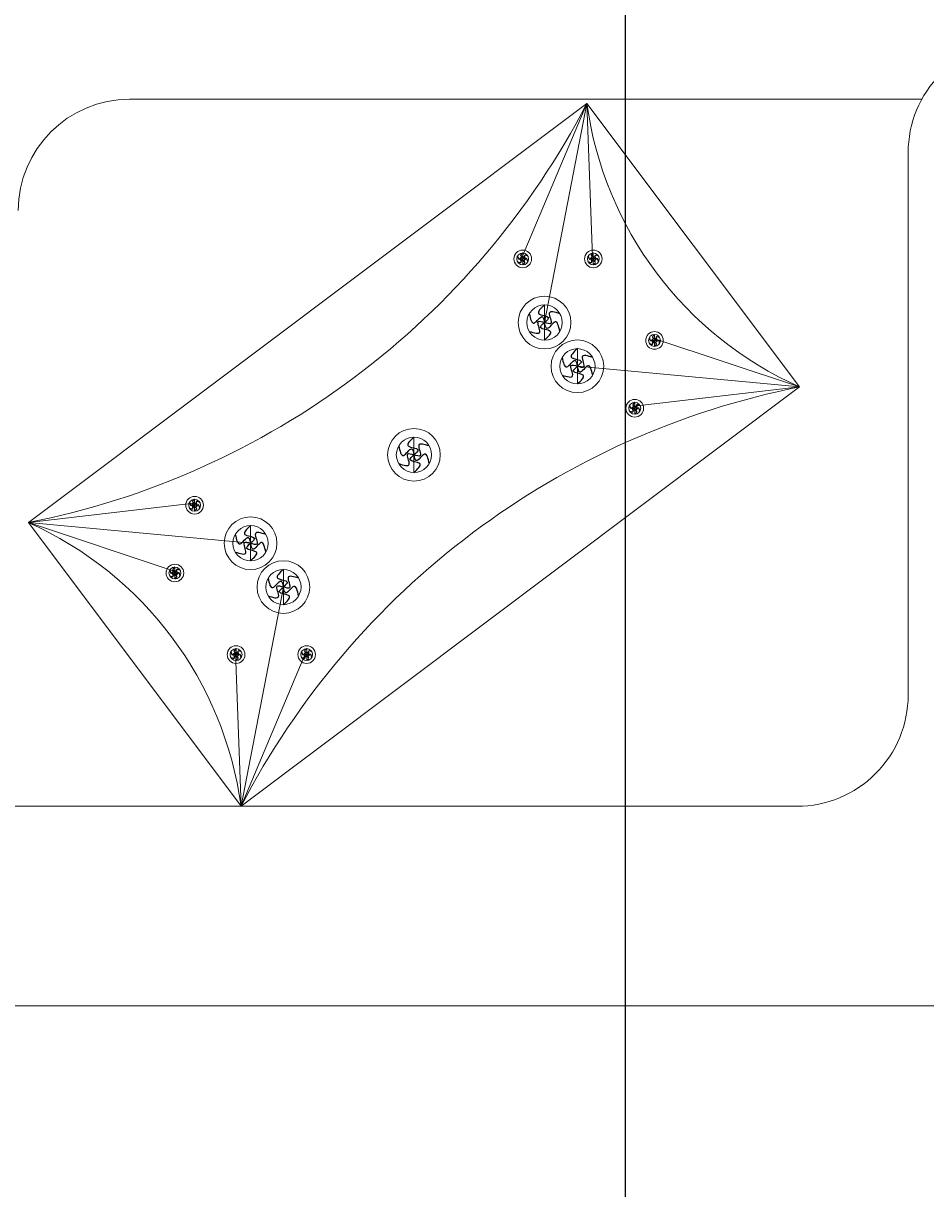
# Model space of a CAD drawing. Units: inches. Extents: x -61 to 1599, y -1316 to 257.
# Tile 107 of 204: x 200 to 224, y -166 to -135. Entities that reach past the tile are written whole.
import ezdxf

# ---------------------------------------------------------------- set-up
doc = ezdxf.new("R2010")
doc.units = ezdxf.units.IN
doc.header["$MEASUREMENT"] = 0
doc.layers.add('A-ANNO-DIMS', color=2, linetype='Continuous', lineweight=18)
doc.layers.add('FURNITURE', color=83, linetype='Continuous', lineweight=18)
doc.layers.add('FUR', color=83, linetype='Continuous')
doc.styles.get("Standard").update_dxf_attribs({"font": 'arial.ttf'})
doc.dimstyles.get("Standard").update_dxf_attribs({"dimtxt": 0.18, "dimasz": 0.18, "dimexe": 0.18, "dimexo": 0.0625, "dimgap": 0.09, "dimtad": 0, "dimtih": 1, "dimtoh": 1, "dimdec": 0, "dimzin": 0, "dimdsep": 46, "dimlunit": 3, "dimtxsty": 'Standard', "dimcen": 0.09, "dimadec": 0, "dimazin": 0, "dimtfac": 1, "dimtdec": 0, "dimtofl": 0, "dimtmove": 0, "dimatfit": 3, "dimfxl": 1, "dimtolj": 1, "dimtzin": 0, "dimarcsym": 0})

# ---------------------------------------------------------------- blocks, each defined once
blk = doc.blocks.new('*U114')
at = {"layer": 'FUR'}
blk.add_open_spline([(0.005, 0.08), (-0.03, 0.048), (-0.098, -0.015), (0.075, -0.018), (0.024, -0.063), (0.005, -0.08)], degree=3, knots=[0, 0, 0, 0, 0.0954578, 0.1898773, 0.2470677, 0.2470677, 0.2470677, 0.2470677], dxfattribs=at)
blk = doc.blocks.new('*U115')
at = {"layer": 'FUR', "transparency": 16777216}
for p, rotation in [((222.173, -79.977), 60), ((222.178, -80.056), 120), ((222.25, -80.092), 180), ((222.312, -79.968), 300), ((222.317, -80.048), 240)]:
    blk.add_blockref('*U114', p, dxfattribs=dict(at, rotation=rotation))
blk.add_blockref('*U114', (222.24, -79.932), dxfattribs=at)
blk = doc.blocks.new('*U116')
at = {"layer": 'FUR'}
blk.add_open_spline([(0.005, 0.08), (-0.03, 0.048), (-0.098, -0.015), (0.075, -0.018), (0.024, -0.063), (0.005, -0.08)], degree=3, knots=[0, 0, 0, 0, 0.0954578, 0.1898773, 0.2470677, 0.2470677, 0.2470677, 0.2470677], dxfattribs=at)
blk = doc.blocks.new('*U117')
at = {"layer": 'FUR', "transparency": 16777216}
for p, rotation in [((222.173, -79.977), 60), ((222.178, -80.056), 120), ((222.25, -80.092), 180), ((222.312, -79.968), 300), ((222.317, -80.048), 240)]:
    blk.add_blockref('*U116', p, dxfattribs=dict(at, rotation=rotation))
blk.add_blockref('*U116', (222.24, -79.932), dxfattribs=at)
blk = doc.blocks.new('*U112')
at = {"layer": 'FUR'}
blk.add_open_spline([(0.005, 0.08), (-0.03, 0.048), (-0.098, -0.015), (0.075, -0.018), (0.024, -0.063), (0.005, -0.08)], degree=3, knots=[0, 0, 0, 0, 0.0954578, 0.1898773, 0.2470677, 0.2470677, 0.2470677, 0.2470677], dxfattribs=at)
blk = doc.blocks.new('*U113')
at = {"layer": 'FUR', "transparency": 16777216}
for p, rotation in [((222.173, -79.977), 60), ((222.178, -80.056), 120), ((222.25, -80.092), 180), ((222.312, -79.968), 300), ((222.317, -80.048), 240)]:
    blk.add_blockref('*U112', p, dxfattribs=dict(at, rotation=rotation))
blk.add_blockref('*U112', (222.24, -79.932), dxfattribs=at)
blk = doc.blocks.new('*U142')
at = {"layer": 'FUR'}
blk.add_open_spline([(0.015, 0.238), (-0.088, 0.143), (-0.292, -0.045), (0.224, -0.053), (0.072, -0.187), (0.015, -0.238)], degree=3, knots=[0, 0, 0, 0, 0.2846533, 0.5662105, 0.736751, 0.736751, 0.736751, 0.736751], dxfattribs=at)
blk = doc.blocks.new('*U143')
at = {"layer": 'FUR', "transparency": 16777216}
blk.add_blockref('*U142', (662.716, -238.357), dxfattribs=at)
for p, rotation in [((662.517, -238.489), 60), ((662.929, -238.463), 300), ((662.944, -238.702), 240), ((662.531, -238.727), 120), ((662.745, -238.833), 180)]:
    blk.add_blockref('*U142', p, dxfattribs=dict(at, rotation=rotation))
blk = doc.blocks.new('*U158')
at = {"layer": 'FUR'}
blk.add_open_spline([(0.015, 0.238), (-0.088, 0.143), (-0.292, -0.045), (0.224, -0.053), (0.072, -0.187), (0.015, -0.238)], degree=3, knots=[0, 0, 0, 0, 0.2846533, 0.5662105, 0.736751, 0.736751, 0.736751, 0.736751], dxfattribs=at)
blk = doc.blocks.new('*U109')
at = {"layer": 'FUR', "transparency": 16777216}
blk.add_blockref('*U158', (662.716, -238.357), dxfattribs=at)
for p, rotation in [((662.517, -238.489), 60), ((662.929, -238.463), 300), ((662.944, -238.702), 240), ((662.531, -238.727), 120), ((662.745, -238.833), 180)]:
    blk.add_blockref('*U158', p, dxfattribs=dict(at, rotation=rotation))
blk = doc.blocks.new('*U110')
at = {"layer": 'FUR'}
blk.add_open_spline([(0.005, 0.08), (-0.03, 0.048), (-0.098, -0.015), (0.075, -0.018), (0.024, -0.063), (0.005, -0.08)], degree=3, knots=[0, 0, 0, 0, 0.0954578, 0.1898773, 0.2470677, 0.2470677, 0.2470677, 0.2470677], dxfattribs=at)
blk = doc.blocks.new('*U111')
at = {"layer": 'FUR', "transparency": 16777216}
for p, rotation in [((222.173, -79.977), 60), ((222.178, -80.056), 120), ((222.25, -80.092), 180), ((222.312, -79.968), 300), ((222.317, -80.048), 240)]:
    blk.add_blockref('*U110', p, dxfattribs=dict(at, rotation=rotation))
blk.add_blockref('*U110', (222.24, -79.932), dxfattribs=at)
blk = doc.blocks.new('*U156')
at = {"layer": 'FUR'}
blk.add_open_spline([(0.015, 0.238), (-0.088, 0.143), (-0.292, -0.045), (0.224, -0.053), (0.072, -0.187), (0.015, -0.238)], degree=3, knots=[0, 0, 0, 0, 0.2846533, 0.5662105, 0.736751, 0.736751, 0.736751, 0.736751], dxfattribs=at)
blk = doc.blocks.new('*U157')
at = {"layer": 'FUR', "transparency": 16777216}
blk.add_blockref('*U156', (662.716, -238.357), dxfattribs=at)
for p, rotation in [((662.517, -238.489), 60), ((662.929, -238.463), 300), ((662.944, -238.702), 240), ((662.531, -238.727), 120), ((662.745, -238.833), 180)]:
    blk.add_blockref('*U156', p, dxfattribs=dict(at, rotation=rotation))
blk = doc.blocks.new('*U120')
at = {"layer": 'FUR'}
blk.add_open_spline([(0.005, 0.08), (-0.03, 0.048), (-0.098, -0.015), (0.075, -0.018), (0.024, -0.063), (0.005, -0.08)], degree=3, knots=[0, 0, 0, 0, 0.0954578, 0.1898773, 0.2470677, 0.2470677, 0.2470677, 0.2470677], dxfattribs=at)
blk = doc.blocks.new('*U121')
at = {"layer": 'FUR', "transparency": 16777216}
for p, rotation in [((222.173, -79.977), 60), ((222.178, -80.056), 120), ((222.25, -80.092), 180), ((222.312, -79.968), 300), ((222.317, -80.048), 240)]:
    blk.add_blockref('*U120', p, dxfattribs=dict(at, rotation=rotation))
blk.add_blockref('*U120', (222.24, -79.932), dxfattribs=at)
blk = doc.blocks.new('*U140')
at = {"layer": 'FUR'}
blk.add_open_spline([(0.015, 0.238), (-0.088, 0.143), (-0.292, -0.045), (0.224, -0.053), (0.072, -0.187), (0.015, -0.238)], degree=3, knots=[0, 0, 0, 0, 0.2846533, 0.5662105, 0.736751, 0.736751, 0.736751, 0.736751], dxfattribs=at)
blk = doc.blocks.new('*U141')
at = {"layer": 'FUR', "transparency": 16777216}
blk.add_blockref('*U140', (662.716, -238.357), dxfattribs=at)
for p, rotation in [((662.517, -238.489), 60), ((662.929, -238.463), 300), ((662.944, -238.702), 240), ((662.531, -238.727), 120), ((662.745, -238.833), 180)]:
    blk.add_blockref('*U140', p, dxfattribs=dict(at, rotation=rotation))
blk = doc.blocks.new('*U135')
at = {"layer": 'FUR'}
blk.add_open_spline([(0.015, 0.238), (-0.088, 0.143), (-0.292, -0.045), (0.224, -0.053), (0.072, -0.187), (0.015, -0.238)], degree=3, knots=[0, 0, 0, 0, 0.2846533, 0.5662105, 0.736751, 0.736751, 0.736751, 0.736751], dxfattribs=at)
blk = doc.blocks.new('*U136')
at = {"layer": 'FUR', "transparency": 16777216}
blk.add_blockref('*U135', (662.716, -238.357), dxfattribs=at)
for p, rotation in [((662.517, -238.489), 60), ((662.929, -238.463), 300), ((662.944, -238.702), 240), ((662.531, -238.727), 120), ((662.745, -238.833), 180)]:
    blk.add_blockref('*U135', p, dxfattribs=dict(at, rotation=rotation))
blk = doc.blocks.new('*U118')
at = {"layer": 'FUR'}
blk.add_open_spline([(0.005, 0.08), (-0.03, 0.048), (-0.098, -0.015), (0.075, -0.018), (0.024, -0.063), (0.005, -0.08)], degree=3, knots=[0, 0, 0, 0, 0.0954578, 0.1898773, 0.2470677, 0.2470677, 0.2470677, 0.2470677], dxfattribs=at)
blk = doc.blocks.new('*U119')
at = {"layer": 'FUR', "transparency": 16777216}
for p, rotation in [((222.173, -79.977), 60), ((222.178, -80.056), 120), ((222.25, -80.092), 180), ((222.312, -79.968), 300), ((222.317, -80.048), 240)]:
    blk.add_blockref('*U118', p, dxfattribs=dict(at, rotation=rotation))
blk.add_blockref('*U118', (222.24, -79.932), dxfattribs=at)
blk = doc.blocks.new('*U138')
at = {"layer": 'FUR'}
blk.add_open_spline([(0.005, 0.08), (-0.03, 0.048), (-0.098, -0.015), (0.075, -0.018), (0.024, -0.063), (0.005, -0.08)], degree=3, knots=[0, 0, 0, 0, 0.0954578, 0.1898773, 0.2470677, 0.2470677, 0.2470677, 0.2470677], dxfattribs=at)
blk = doc.blocks.new('*U139')
at = {"layer": 'FUR', "transparency": 16777216}
for p, rotation in [((222.173, -79.977), 60), ((222.178, -80.056), 120), ((222.25, -80.092), 180), ((222.312, -79.968), 300), ((222.317, -80.048), 240)]:
    blk.add_blockref('*U138', p, dxfattribs=dict(at, rotation=rotation))
blk.add_blockref('*U138', (222.24, -79.932), dxfattribs=at)
blk = doc.blocks.new('*U122')
at = {"layer": 'FUR'}
blk.add_open_spline([(0.005, 0.08), (-0.03, 0.048), (-0.098, -0.015), (0.075, -0.018), (0.024, -0.063), (0.005, -0.08)], degree=3, knots=[0, 0, 0, 0, 0.0954578, 0.1898773, 0.2470677, 0.2470677, 0.2470677, 0.2470677], dxfattribs=at)
blk = doc.blocks.new('*U137')
at = {"layer": 'FUR', "transparency": 16777216}
for p, rotation in [((222.173, -79.977), 60), ((222.178, -80.056), 120), ((222.25, -80.092), 180), ((222.312, -79.968), 300), ((222.317, -80.048), 240)]:
    blk.add_blockref('*U122', p, dxfattribs=dict(at, rotation=rotation))
blk.add_blockref('*U122', (222.24, -79.932), dxfattribs=at)
blk = doc.blocks.new('SOFA-THREE-SEAT')
for p, q in [((78.369, 24.442), (57, 24.442)), ((69.336, 24.333), (67.586, 20.192)), ((69.336, 24.333), (68.194, 18.423)), ((69.336, 24.333), (69.49, 20.192)), ((67.605, 20.139), (67.605, 20.299)), ((67.605, 20.139), (67.605, 19.979)), ((69.509, 20.139), (69.509, 20.299)), ((69.509, 20.139), (69.509, 19.979)), ((68.194, 18.423), (68.194, 18.899)), ((68.194, 18.423), (68.194, 17.946)), ((75.074, 16.687), (71.14, 17.993)), ((71.159, 17.94), (71.159, 18.1)), ((71.159, 17.94), (71.159, 17.78)), ((69.079, 17.243), (69.079, 17.719)), ((75.074, 16.687), (69.079, 17.243)), ((69.079, 17.243), (69.079, 16.766)), ((75.074, 16.687), (70.608, 16.164)), ((70.627, 16.112), (70.627, 16.272)), ((70.627, 16.112), (70.627, 15.952)), ((64.672, 14.857), (64.672, 15.334)), ((64.672, 14.857), (64.672, 14.381)), ((54.271, 13.028), (58.736, 13.551)), ((58.756, 13.498), (58.756, 13.658)), ((58.756, 13.498), (58.756, 13.338)), ((54.271, 13.028), (60.265, 12.472)), ((54.271, 13.028), (58.204, 11.722)), ((60.265, 12.472), (60.265, 12.949)), ((60.265, 12.472), (60.265, 11.996)), ((58.224, 11.67), (58.224, 11.83)), ((58.224, 11.67), (58.224, 11.51)), ((61.15, 11.292), (61.15, 11.769)), ((60.009, 5.382), (61.15, 11.292)), ((61.15, 11.292), (61.15, 10.816)), ((60.009, 5.382), (59.854, 9.523)), ((59.874, 9.471), (59.874, 9.631)), ((59.874, 9.471), (59.874, 9.311)), ((60.009, 5.382), (61.759, 9.523)), ((61.778, 9.471), (61.778, 9.631)), ((61.778, 9.471), (61.778, 9.311))]:
    blk.add_line(p, q)
blk.add_lwpolyline([(78, 8.382), (78, 23, -0.414214), (81, 26), (81, 26, -0.414214), (84, 23), (84, 3, -0.414214), (81, 0), (3, 0, -0.414214), (0, 3), (0, 23, -0.414214), (3, 26), (3, 26, -0.414214), (6, 23), (6, 8.382, 0.414214), (9, 5.382), (75, 5.382, 0.414214)], format="xyb", close=True)
blk.add_lwpolyline([(54.271, 13.028), (69.336, 24.333), (75.074, 16.687), (60.009, 5.382)], close=True)
for centre, radius in [((67.605, 20.139), 0.238), ((67.605, 20.139), 0.16), ((69.509, 20.139), 0.238), ((69.509, 20.139), 0.16), ((68.194, 18.423), 0.71), ((68.194, 18.423), 0.476), ((69.079, 17.243), 0.71), ((71.159, 17.94), 0.238), ((71.159, 17.94), 0.16), ((69.079, 17.243), 0.476), ((70.627, 16.112), 0.238), ((70.627, 16.112), 0.16), ((64.672, 14.857), 0.71), ((64.672, 14.857), 0.476), ((58.756, 13.498), 0.238), ((58.756, 13.498), 0.16), ((60.265, 12.472), 0.71), ((60.265, 12.472), 0.476), ((61.15, 11.292), 0.71), ((58.224, 11.67), 0.238), ((58.224, 11.67), 0.16), ((61.15, 11.292), 0.476), ((59.874, 9.471), 0.238), ((59.874, 9.471), 0.16), ((61.778, 9.471), 0.238), ((61.778, 9.471), 0.16)]:
    blk.add_circle(centre, radius)
for centre, radius, start, end in [((57, 21.442), 3, 90, 180), ((50.048, 34.345), 21.731, 281.2044, 332.5684), ((79.062, 25.656), 9.816, 187.747, 246.0258), ((79.296, -4.63), 21.731, 101.2044, 152.5684), ((50.282, 4.059), 9.816, 7.747, 66.0258)]:
    blk.add_arc(centre, radius, start, end)
at = {"rotation": 180}
for name, p in [('*U121', (289.85, -59.873)), ('*U119', (291.754, -59.873)), ('*U141', (730.924, -220.172)), ('*U137', (293.404, -62.072)), ('*U136', (731.81, -221.352)), ('*U139', (292.872, -63.9)), ('*U157', (727.402, -223.738)), ('*U117', (281.001, -66.514)), ('*U143', (722.995, -226.123)), ('*U115', (280.469, -68.342)), ('*U109', (723.88, -227.303)), ('*U113', (282.119, -70.541)), ('*U111', (284.023, -70.541))]:
    blk.add_blockref(name, p, dxfattribs=at)
blk = doc.blocks.new('*D670')
at = {"layer": 'A-ANNO-DIMS', "color": 0, "lineweight": -2, "transparency": 16777216}
for p, q in [((145.375, -161.442), (145.375, -174.159)), ((229.375, -161.442), (229.375, -174.159)), ((145.555, -173.979), (186.47, -173.979)), ((229.195, -173.979), (188.279, -173.979))]:
    blk.add_line(p, q, dxfattribs=at)
at = {"layer": 'A-ANNO-DIMS', "color": 0, "transparency": 16777216}
for points in [[(145.555, -173.949), (145.555, -174.009), (145.375, -173.979)], [(229.195, -173.949), (229.195, -174.009), (229.375, -173.979)]]:
    blk.add_solid(points, dxfattribs=at)
at = {"layer": 'DEFPOINTS', "color": 0, "transparency": 16777216}
for p in [(145.375, -161.379), (229.375, -161.379), (229.375, -173.979)]:
    blk.add_point(p, dxfattribs=at)
at = {"layer": 'A-ANNO-DIMS', "color": 0, "transparency": 16777216, "insert": (187.375, -173.979), "char_height": 0.18, "attachment_point": 5}
blk.add_mtext('\\A1;SOFA 84 TYP.', dxfattribs=at)
blk = doc.blocks.new('*D687')
at = {"layer": 'A-ANNO-DIMS', "color": 0, "lineweight": -2, "transparency": 16777216}
for p, q in [((289.418, 181.677), (-61.077, 181.677)), ((-60.897, 181.497), (-60.897, -528.952)), ((-60.897, -1239.765), (-60.897, -529.316)), ((319.64, -1239.945), (-61.077, -1239.945))]:
    blk.add_line(p, q, dxfattribs=at)
at = {"layer": 'A-ANNO-DIMS', "color": 0, "transparency": 16777216}
for points in [[(-60.927, 181.497), (-60.867, 181.497), (-60.897, 181.677)], [(-60.927, -1239.765), (-60.867, -1239.765), (-60.897, -1239.945)]]:
    blk.add_solid(points, dxfattribs=at)
at = {"layer": 'DEFPOINTS', "color": 0, "transparency": 16777216}
for p in [(289.481, 181.677), (-60.897, -1239.945), (319.703, -1239.945)]:
    blk.add_point(p, dxfattribs=at)
at = {"layer": 'A-ANNO-DIMS', "color": 0, "transparency": 16777216, "insert": (-60.897, -529.134), "char_height": 0.18, "attachment_point": 5}
blk.add_mtext('\\A1;1421.6', dxfattribs=at)
blk = doc.blocks.new('*D701')
at = {"layer": 'A-ANNO-DIMS', "color": 0, "lineweight": -2, "transparency": 16777216}
for p, q in [((215.752, -616.882), (215.752, 257.457)), ((252.882, -616.882), (252.882, 257.457)), ((215.932, 257.277), (233.924, 257.277)), ((252.702, 257.277), (234.711, 257.277))]:
    blk.add_line(p, q, dxfattribs=at)
at = {"layer": 'A-ANNO-DIMS', "color": 0, "transparency": 16777216}
for points in [[(215.932, 257.307), (215.932, 257.247), (215.752, 257.277)], [(252.702, 257.307), (252.702, 257.247), (252.882, 257.277)]]:
    blk.add_solid(points, dxfattribs=at)
at = {"layer": 'DEFPOINTS', "color": 0, "transparency": 16777216}
for p in [(252.882, 257.277), (215.752, -616.945), (252.882, -616.945)]:
    blk.add_point(p, dxfattribs=at)
at = {"layer": 'A-ANNO-DIMS', "color": 0, "transparency": 16777216, "insert": (234.317, 257.277), "char_height": 0.18, "attachment_point": 5}
blk.add_mtext('\\A1;37.13', dxfattribs=at)

msp = doc.modelspace()

# ---------------------------------------------------------------- block references
at = {"layer": 'FURNITURE'}
msp.add_blockref('SOFA-THREE-SEAT', (145.375, -161.379), dxfattribs=at)

# ---------------------------------------------------------------- dimensions: what is measured, and where the dimension line sits
at = {"layer": 'A-ANNO-DIMS'}
dim = msp.add_linear_dim(base=(252.8825, 257.2771), p1=(215.7521, -616.9446), p2=(252.8825, -616.9446), dimstyle='Standard', override={"dimdec": 2, "dimlfac": 1, "dimrnd": 0, "dimzin": 0, "dimdsep": 46, "dimlunit": 2}, dxfattribs=at)
dim.commit()
dim.dimension.update_dxf_attribs({"geometry": '*D701', "text_midpoint": (234.3173, 257.2771)})
dim = msp.add_linear_dim(base=(-60.8972, -1239.9446), p1=(289.4807, 181.6771), p2=(319.7028, -1239.9446), angle=90, dimstyle='Standard', override={"dimdec": 1, "dimlfac": 1, "dimrnd": 0, "dimzin": 0, "dimdsep": 46, "dimlunit": 2}, dxfattribs=at)
dim.commit()
dim.dimension.update_dxf_attribs({"geometry": '*D687', "text_midpoint": (-60.8972, -529.1337)})
dim = msp.add_linear_dim(base=(229.3746, -173.9792), p1=(145.3746, -161.3792), p2=(229.3746, -161.3792), text='SOFA <> TYP.', dimstyle='Standard', override={"dimdec": 0, "dimlfac": 1, "dimrnd": 0, "dimzin": 0, "dimdsep": 46, "dimlunit": 2}, dxfattribs=at)
dim.commit()
dim.dimension.update_dxf_attribs({"geometry": '*D670', "text_midpoint": (187.3746, -173.9792)})

doc.saveas('drawing.dxf')
